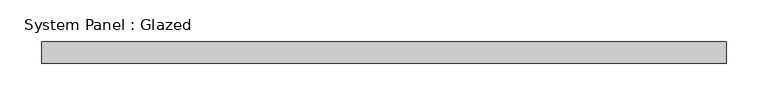
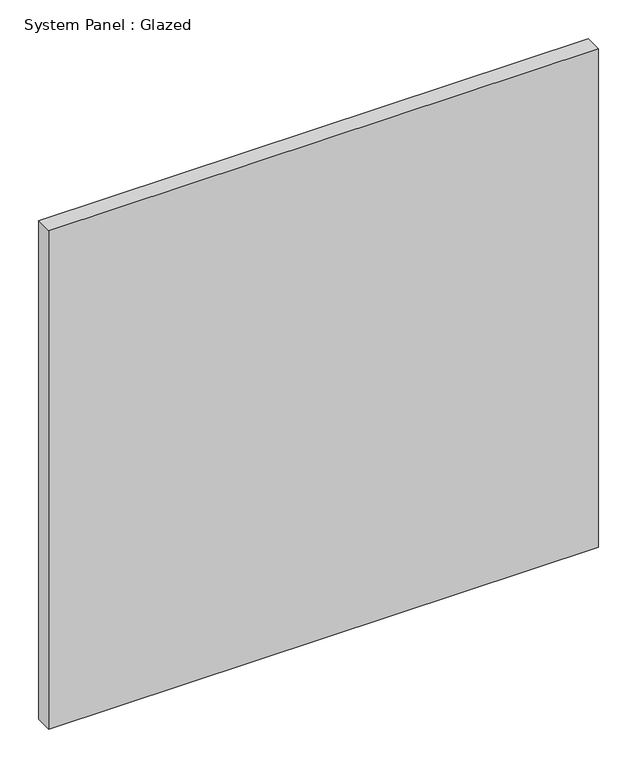
"""IFC4 building model written with IfcOpenShell, lengths in millimetres: plate geometry, System Panel : Glazed."""

from ifc_helpers import new_model, si_unit, origin, origin_with_axes, place, context, project, spatial, polyline, outline, extrude, source, transform, mapped, element, save


def system_panel_glazed_5425f88c(model_context):
    return source(origin(), model_context, "Body", "SweptSolid", [
        extrude(outline(polyline([(409.575, 19.05), (-409.575, 19.05), (-409.575, 44.45), (409.575, 44.45), (409.575, 19.05)])), origin_with_axes(), (0.0, 0.0, 1.0), 785.0152244),
    ])


if __name__ == "__main__":
    model = new_model("IFC4")
    model_context = context("Model", 3, world=origin())
    ifc_project = project(units=[si_unit("LENGTHUNIT", "METRE", prefix="MILLI")], contexts=[model_context])
    site = spatial("IfcSite", under=ifc_project)
    building = spatial("IfcBuilding", under=site)
    placement = place(None, origin())
    system_panel_glazed_shape = system_panel_glazed_5425f88c(model_context)
    element("IfcPlate", 1, ObjectType="System Panel : Glazed", at=placement, inside=building, context=model_context, shape_type="MappedRepresentation", body=[
        mapped(system_panel_glazed_shape, transform((0.0, 0.0, 0.0), x_axis=(1.0, 0.0, 0.0), y_axis=(0.0, 1.0, 0.0), z_axis=(0.0, 0.0, 1.0))),
    ])
    save(model, "model.ifc")

# Revit data of these elements
# Type "System Panel : Glazed"
#   Construction Type Id = "GSP4R"
#   Analytic Construction = "1/8 in Pilkington single glazing"
#   Visual Light Transmittance = 0.9
#   Solar Heat Gain Coefficient = 0.86
#   Heat Transfer Coefficient (U) = 1.18115 BTU/(h·ft²·°F)
#   Define Thermal Properties by = 1
# Element 1 (IfcPlate, "System Panel : Glazed")
#   Materials on its faces: "Glass"
# Materials
#   "Glass": class "Glass", colour RGB 0 128 192, transparency 0.75, Description = "Soda Lime Glass", Cost = 0
